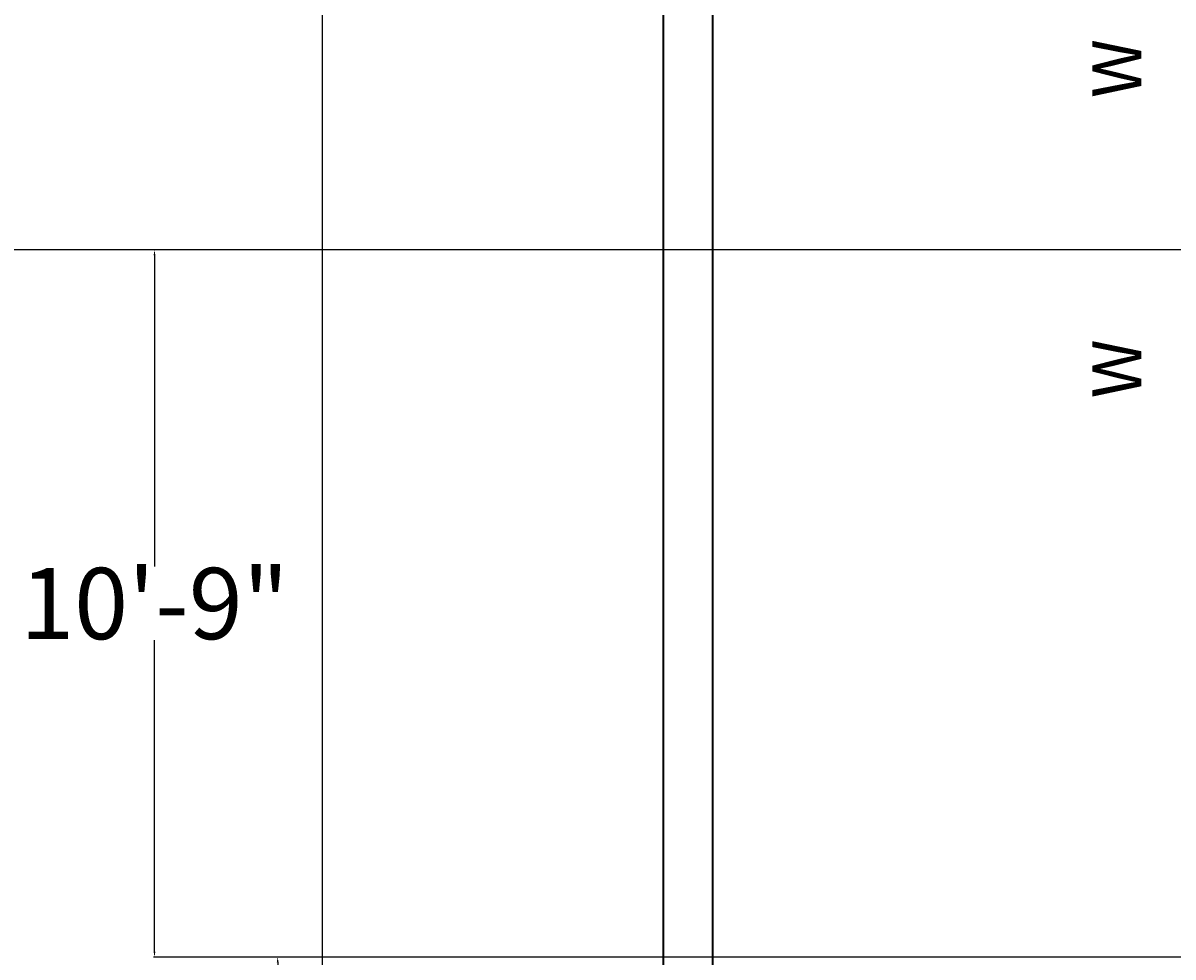
# Model space of a CAD drawing. Units: inches. Extents: x -364 to 705, y -52 to 1250.
# Tile 5 of 34: x -181 to 29, y 323 to 494. Entities that reach past the tile are written whole.
import ezdxf

# ---------------------------------------------------------------- set-up
doc = ezdxf.new("R2010")
doc.units = ezdxf.units.IN
doc.header["$MEASUREMENT"] = 0
for name, color, linetype, lineweight in [('A-ANNO-DIMS', 4, 'Continuous', 18), ('A-ANNO-IDEN', 1, 'Continuous', 18), ('C-WALL', 41, 'Continuous', 35)]:
    doc.layers.add(name, color=color, linetype=linetype, lineweight=lineweight)
doc.styles.get("Standard").update_dxf_attribs({"font": 'arial.ttf'})
doc.dimstyles.get("Standard").update_dxf_attribs({"dimtxt": 1, "dimasz": 1, "dimexe": 0.18, "dimexo": 0.0625, "dimgap": 0.09, "dimtad": 0, "dimtih": 1, "dimtoh": 1, "dimdec": 0, "dimzin": 0, "dimdsep": 46, "dimlunit": 3, "dimtxsty": 'Standard', "dimcen": 0.09, "dimadec": 0, "dimazin": 0, "dimtfac": 1, "dimtdec": 0, "dimtofl": 0, "dimtmove": 0, "dimatfit": 3, "dimfxl": 1, "dimtolj": 1, "dimtzin": 0, "dimarcsym": 0})

# ---------------------------------------------------------------- blocks, each defined once
blk = doc.blocks.new('*D19')
at = {"layer": 'A-ANNO-DIMS', "color": 0, "lineweight": -2, "transparency": 16777216}
for p, q in [((28.52, 986.11), (-248.33, 986.11)), ((-248.15, 985.11), (-248.15, 574.22)), ((-248.15, 149.87), (-248.15, 560.77)), ((28.52, 148.87), (-248.33, 148.87))]:
    blk.add_line(p, q, dxfattribs=at)
at = {"layer": 'A-ANNO-DIMS', "color": 0, "transparency": 16777216}
for points in [[(-248.32, 985.11), (-247.99, 985.11), (-248.15, 986.11)], [(-248.32, 149.87), (-247.99, 149.87), (-248.15, 148.87)]]:
    blk.add_solid(points, dxfattribs=at)
at = {"layer": 'Defpoints', "color": 0, "transparency": 16777216}
for p in [(28.58, 986.11), (-248.15, 148.87), (28.58, 148.87)]:
    blk.add_point(p, dxfattribs=at)
at = {"layer": 'A-ANNO-DIMS', "color": 0, "transparency": 16777216, "insert": (-248.15, 567.49), "char_height": 1, "attachment_point": 5}
blk.add_mtext('\\A1;{\\H13x;69\'-9"}', dxfattribs=at)
blk = doc.blocks.new('*D28')
at = {"layer": 'A-ANNO-DIMS', "color": 0, "lineweight": -2, "transparency": 16777216}
for p, q in [((37.52, 323.11), (-135.02, 323.11)), ((-134.84, 322.11), (-134.84, 242.84)), ((-134.84, 150.11), (-134.84, 229.39)), ((37.52, 149.11), (-135.02, 149.11))]:
    blk.add_line(p, q, dxfattribs=at)
at = {"layer": 'A-ANNO-DIMS', "color": 0, "transparency": 16777216}
for points in [[(-135.01, 322.11), (-134.67, 322.11), (-134.84, 323.11)], [(-135.01, 150.11), (-134.67, 150.11), (-134.84, 149.11)]]:
    blk.add_solid(points, dxfattribs=at)
at = {"layer": 'Defpoints', "color": 0, "transparency": 16777216}
for p in [(-134.84, 323.11), (37.58, 323.11), (37.58, 149.11)]:
    blk.add_point(p, dxfattribs=at)
at = {"layer": 'A-ANNO-DIMS', "color": 0, "transparency": 16777216, "insert": (-134.84, 236.11), "char_height": 1, "attachment_point": 5}
blk.add_mtext('\\A1;{\\H13x;14\'-6"}', dxfattribs=at)
blk = doc.blocks.new('*D29')
at = {"layer": 'A-ANNO-DIMS', "color": 0, "lineweight": -2, "transparency": 16777216}
for p, q in [((37.52, 452.11), (-157.5, 452.11)), ((-157.32, 451.11), (-157.32, 394.34)), ((-157.32, 324.11), (-157.32, 380.89)), ((28.52, 323.11), (-157.5, 323.11))]:
    blk.add_line(p, q, dxfattribs=at)
at = {"layer": 'A-ANNO-DIMS', "color": 0, "transparency": 16777216}
for points in [[(-157.49, 451.11), (-157.16, 451.11), (-157.32, 452.11)], [(-157.49, 324.11), (-157.16, 324.11), (-157.32, 323.11)]]:
    blk.add_solid(points, dxfattribs=at)
at = {"layer": 'Defpoints', "color": 0, "transparency": 16777216}
for p in [(-157.32, 452.11), (37.58, 452.11), (28.58, 323.11)]:
    blk.add_point(p, dxfattribs=at)
at = {"layer": 'A-ANNO-DIMS', "color": 0, "transparency": 16777216, "insert": (-157.32, 387.61), "char_height": 1, "attachment_point": 5}
blk.add_mtext('\\A1;{\\H13x;10\'-9"}', dxfattribs=at)
blk = doc.blocks.new('*D30')
at = {"layer": 'A-ANNO-DIMS', "color": 0, "lineweight": -2, "transparency": 16777216}
for p, q in [((28.52, 578.1), (-188.97, 578.1)), ((-188.79, 577.1), (-188.79, 521.83)), ((-188.79, 453.11), (-188.79, 508.38)), ((28.52, 452.11), (-188.97, 452.11))]:
    blk.add_line(p, q, dxfattribs=at)
at = {"layer": 'A-ANNO-DIMS', "color": 0, "transparency": 16777216}
for points in [[(-188.96, 577.1), (-188.63, 577.1), (-188.79, 578.1)], [(-188.96, 453.11), (-188.63, 453.11), (-188.79, 452.11)]]:
    blk.add_solid(points, dxfattribs=at)
at = {"layer": 'Defpoints', "color": 0, "transparency": 16777216}
for p in [(-188.79, 578.1), (28.58, 578.1), (28.58, 452.11)]:
    blk.add_point(p, dxfattribs=at)
at = {"layer": 'A-ANNO-DIMS', "color": 0, "transparency": 16777216, "insert": (-188.79, 515.11), "char_height": 1, "attachment_point": 5}
blk.add_mtext('\\A1;{\\H13x;10\'-6"}', dxfattribs=at)
blk = doc.blocks.new('*D76')
at = {"layer": 'A-ANNO-DIMS', "color": 0, "lineweight": -2, "transparency": 16777216}
for p, q in [((28.52, 986.11), (-126.85, 986.11)), ((-126.67, 985.11), (-126.67, 499.22)), ((-126.67, 12.11), (-126.67, 498.01)), ((28.52, 11.11), (-126.85, 11.11))]:
    blk.add_line(p, q, dxfattribs=at)
at = {"layer": 'A-ANNO-DIMS', "color": 0, "transparency": 16777216}
for points in [[(-126.84, 985.11), (-126.5, 985.11), (-126.67, 986.11)], [(-126.84, 12.11), (-126.5, 12.11), (-126.67, 11.11)]]:
    blk.add_solid(points, dxfattribs=at)
at = {"layer": 'Defpoints', "color": 0, "transparency": 16777216}
for p in [(-126.67, 986.11), (28.58, 986.11), (28.58, 11.11)]:
    blk.add_point(p, dxfattribs=at)
at = {"layer": 'A-ANNO-DIMS', "color": 0, "transparency": 16777216, "insert": (-126.67, 498.61), "char_height": 1, "attachment_point": 5}
blk.add_mtext('\\A1;81\'-3"', dxfattribs=at)

msp = doc.modelspace()

# ---------------------------------------------------------------- linework, layer by layer
at = {"layer": 'C-WALL'}
for p, q in [((-64.42, 11.11), (-64.42, 1079.11)), ((-55.42, 11.11), (-55.42, 1070.11))]:
    msp.add_line(p, q, dxfattribs=at)

# ---------------------------------------------------------------- texts
at = {"layer": 'A-ANNO-IDEN', "char_height": 9, "attachment_point": 1, "rotation": 90}
for insert in [(13.83, 479.82), (13.83, 425.03)]:
    msp.add_mtext_dynamic_manual_height_columns('W', width=31.4151, gutter_width=1, heights=[0], dxfattribs=dict(at, insert=insert))

# ---------------------------------------------------------------- dimensions: what is measured, and where the dimension line sits
at = {"layer": 'A-ANNO-DIMS'}
for base, p1, p2, picture, middle in [((-248.15, 148.87), (28.58, 986.11), (28.58, 148.87), '*D19', (-248.15, 567.49)), ((-188.79, 578.1), (28.58, 452.11), (28.58, 578.1), '*D30', (-188.79, 515.11)), ((-157.32, 452.11), (28.58, 323.11), (37.58, 452.11), '*D29', (-157.32, 387.61)), ((-134.84, 323.11), (37.58, 149.11), (37.58, 323.11), '*D28', (-134.84, 236.11))]:
    dim = msp.add_linear_dim(base=base, p1=p1, p2=p2, angle=90, text='{\\H13x;<>}', dimstyle='Standard', override={"dimclrd": 0, "dimclre": 0, "dimclrt": 0}, dxfattribs=at)
    dim.commit()
    dim.dimension.update_dxf_attribs({"geometry": picture, "text_midpoint": middle})
dim = msp.add_linear_dim(base=(-126.67, 986.11), p1=(28.58, 11.11), p2=(28.58, 986.11), angle=90, dimstyle='Standard', override={"dimdec": 1, "dimlfac": 1, "dimrnd": 0, "dimzin": 1, "dimdsep": 46, "dimlunit": 4, "dimfrac": 2}, dxfattribs=at)
dim.commit()
dim.dimension.update_dxf_attribs({"geometry": '*D76', "text_midpoint": (-126.67, 498.61)})

doc.saveas('drawing.dxf')
